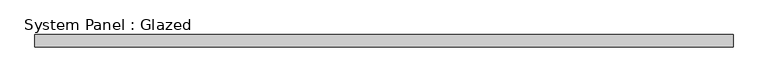
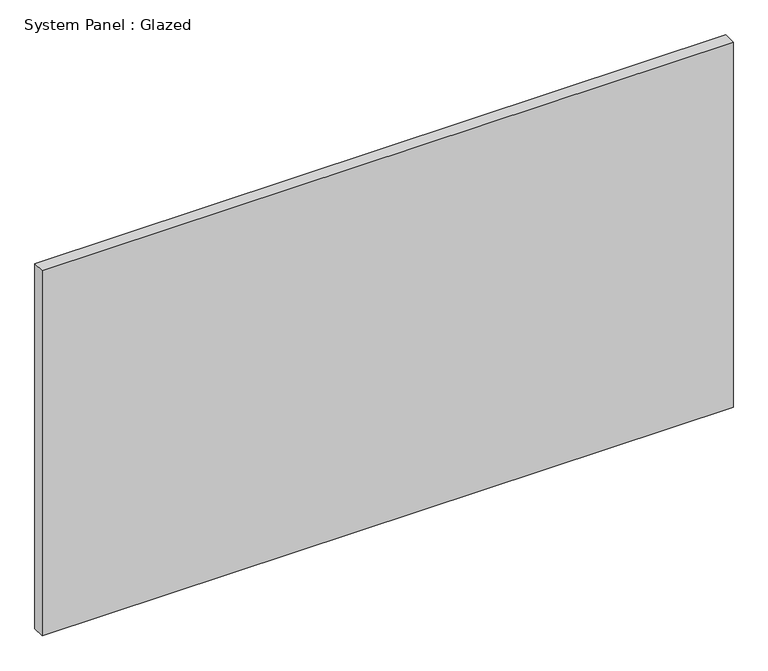
"""IFC4 building model written with IfcOpenShell, lengths in millimetres: plate geometry, System Panel : Glazed."""

from ifc_helpers import new_model, si_unit, origin, origin_with_axes, place, context, project, spatial, polyline, outline, extrude, source, transform, mapped, element, save


def system_panel_glazed_27716cba(model_context):
    return source(origin(), model_context, "Body", "SweptSolid", [
        extrude(outline(polyline([(704.8499999, 19.05), (-704.8499999, 19.05), (-704.8499999, 44.45), (704.8499999, 44.45), (704.8499999, 19.05)])), origin_with_axes(), (0.0, 0.0, 1.0), 787.4),
    ])


if __name__ == "__main__":
    model = new_model("IFC4")
    model_context = context("Model", 3, world=origin())
    ifc_project = project(units=[si_unit("LENGTHUNIT", "METRE", prefix="MILLI")], contexts=[model_context])
    site = spatial("IfcSite", under=ifc_project)
    building = spatial("IfcBuilding", under=site)
    placement = place(None, origin())
    system_panel_glazed_shape = system_panel_glazed_27716cba(model_context)
    element("IfcPlate", 1, ObjectType="System Panel : Glazed", at=placement, inside=building, context=model_context, shape_type="MappedRepresentation", body=[
        mapped(system_panel_glazed_shape, transform((0.0, 0.0, 0.0), x_axis=(1.0, 0.0, 0.0), y_axis=(0.0, 1.0, 0.0), z_axis=(0.0, 0.0, 1.0))),
    ])
    save(model, "model.ifc")

# Revit data of these elements
# Type "System Panel : Glazed"
#   Construction Type Id = "GSP4R"
#   Analytic Construction = "1/8 in Pilkington single glazing"
#   Visual Light Transmittance = 0.9
#   Solar Heat Gain Coefficient = 0.86
#   Heat Transfer Coefficient (U) = 1.18115 BTU/(h·ft²·°F)
#   Define Thermal Properties by = 1
# Element 1 (IfcPlate, "System Panel : Glazed")
#   Materials on its faces: "Glass"
# Materials
#   "Glass": class "Glass", colour RGB 0 128 192, transparency 0.75, Description = "Soda Lime Glass", Cost = 0
